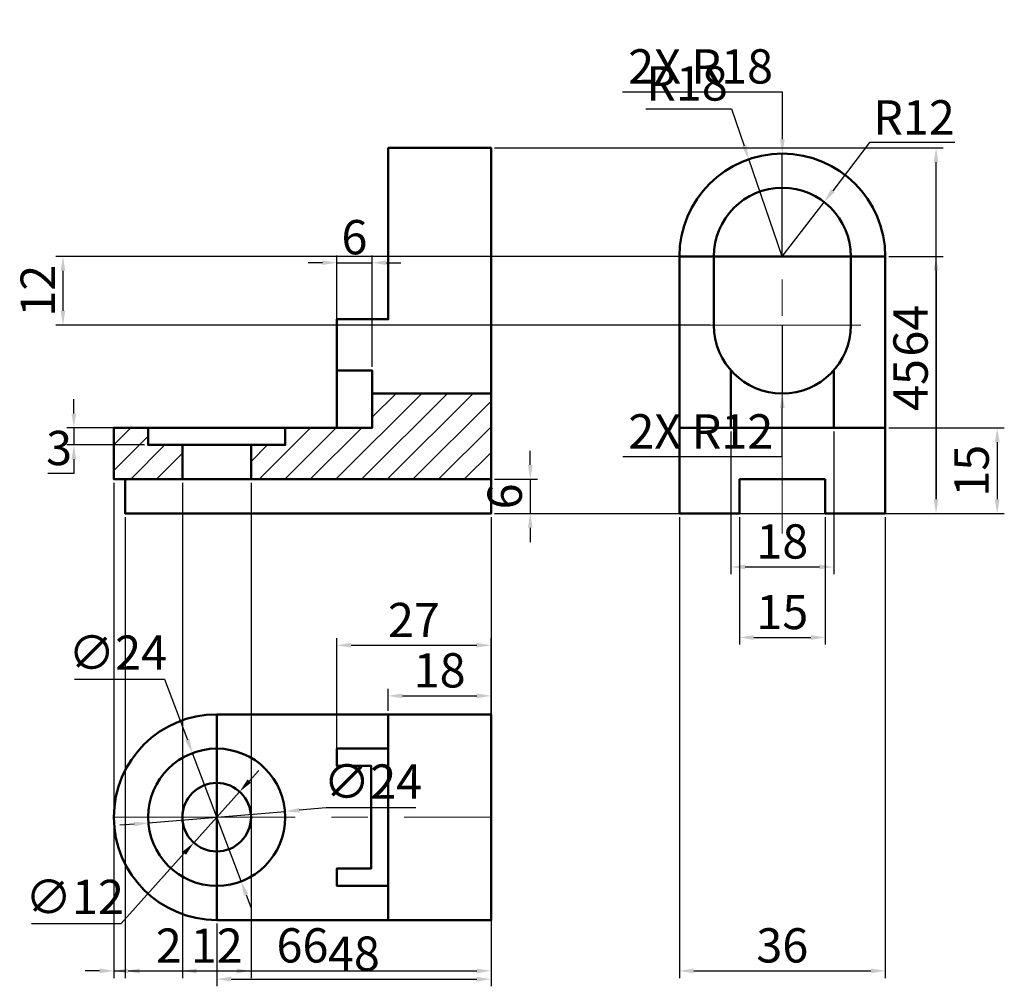
# Model space of a CAD drawing. Units: millimetres. Extents: x 1 to 173, y 26 to 195.
import ezdxf

# ---------------------------------------------------------------- set-up
doc = ezdxf.new("R2010")
doc.units = ezdxf.units.MM
doc.linetypes.add('CENTER', pattern=[50.8, 31.75, -6.35, 6.35, -6.35])
for name, color, linetype, lineweight in [('M-CNTR', 4, 'CENTER', 18), ('M-DIMS', 2, 'Continuous', 25), ('M-HATC', 8, 'Continuous', 18), ('M-OUTL', 7, 'Continuous', 50)]:
    doc.layers.add(name, color=color, linetype=linetype, lineweight=lineweight)
doc.styles.get("Standard").update_dxf_attribs({"font": 'arial.ttf'})
doc.dimstyles.new('ISO-25', dxfattribs={"dimtxt": 6, "dimasz": 2.5, "dimexe": 1.25, "dimexo": 0.625, "dimtad": 1, "dimtoh": 1, "dimdec": 0, "dimtxsty": 'Standard', "dimcen": 2.5, "dimadec": 0, "dimazin": 0, "dimtfac": 1, "dimtdec": 0, "dimtmove": 0, "dimatfit": 3, "dimfxl": 1, "dimarcsym": 0})

# ---------------------------------------------------------------- blocks, each defined once
blk = doc.blocks.new('*D1')
at = {"layer": 'Defpoints', "color": 0, "transparency": 16777216}
for p in [(62.71, 152.66), (56.52, 133.82), (62.71, 133.82)]:
    blk.add_point(p, dxfattribs=at)
at = {"layer": 'M-DIMS', "color": 0, "lineweight": -2, "transparency": 16777216}
for p, q in [((56.52, 134.44), (56.52, 153.91)), ((62.71, 134.44), (62.71, 153.91)), ((54.02, 152.66), (51.52, 152.66)), ((56.52, 152.66), (62.71, 152.66)), ((65.21, 152.66), (67.71, 152.66))]:
    blk.add_line(p, q, dxfattribs=at)
at = {"layer": 'M-DIMS', "color": 0, "transparency": 16777216}
for points in [[(54.02, 153.08), (54.02, 152.25), (56.52, 152.66)], [(65.21, 153.08), (65.21, 152.25), (62.71, 152.66)]]:
    blk.add_solid(points, dxfattribs=at)
at = {"layer": 'M-DIMS', "color": 0, "transparency": 16777216, "insert": (59.61, 156.35), "char_height": 6, "attachment_point": 5}
blk.add_mtext('6', dxfattribs=at)
blk = doc.blocks.new('*D2')
at = {"layer": 'Defpoints', "color": 0, "transparency": 16777216}
for p in [(83.52, 114.76), (83.52, 108.76), (90.38, 108.76)]:
    blk.add_point(p, dxfattribs=at)
at = {"layer": 'M-DIMS', "color": 0, "lineweight": -2, "transparency": 16777216}
for p, q in [((90.38, 117.26), (90.38, 119.76)), ((84.15, 114.76), (91.63, 114.76)), ((90.38, 114.76), (90.38, 108.76)), ((84.15, 108.76), (91.63, 108.76)), ((90.38, 106.26), (90.38, 103.76))]:
    blk.add_line(p, q, dxfattribs=at)
at = {"layer": 'M-DIMS', "color": 0, "transparency": 16777216}
for points in [[(89.96, 117.26), (90.79, 117.26), (90.38, 114.76)], [(89.96, 106.26), (90.79, 106.26), (90.38, 108.76)]]:
    blk.add_solid(points, dxfattribs=at)
at = {"layer": 'M-DIMS', "color": 0, "transparency": 16777216, "insert": (86.69, 111.76), "char_height": 6, "attachment_point": 5, "rotation": 90}
blk.add_mtext('6', dxfattribs=at)
blk = doc.blocks.new('*D3')
at = {"layer": 'Defpoints', "color": 0, "transparency": 16777216}
for p in [(23.52, 123.76), (10.53, 120.76), (23.52, 120.76)]:
    blk.add_point(p, dxfattribs=at)
at = {"layer": 'M-DIMS', "color": 0, "lineweight": -2, "transparency": 16777216}
for p, q in [((10.53, 126.26), (10.53, 128.76)), ((22.9, 123.76), (9.28, 123.76)), ((10.53, 123.76), (10.53, 120.76)), ((22.9, 120.76), (9.28, 120.76)), ((10.53, 118.26), (10.53, 115.76)), ((10.53, 115.76), (5.97, 115.76))]:
    blk.add_line(p, q, dxfattribs=at)
at = {"layer": 'M-DIMS', "color": 0, "transparency": 16777216}
for points in [[(10.11, 126.26), (10.94, 126.26), (10.53, 123.76)], [(10.11, 118.26), (10.94, 118.26), (10.53, 120.76)]]:
    blk.add_solid(points, dxfattribs=at)
at = {"layer": 'M-DIMS', "color": 0, "transparency": 16777216, "insert": (7.94, 119.45), "char_height": 6, "attachment_point": 5}
blk.add_mtext('3', dxfattribs=at)
blk = doc.blocks.new('*D4')
at = {"layer": 'Defpoints', "color": 0, "transparency": 16777216}
for p in [(128.62, 170.77), (134.48, 153.75)]:
    blk.add_point(p, dxfattribs=at)
at = {"layer": 'M-DIMS', "color": 0, "lineweight": -2, "transparency": 16777216}
for p, q in [((110.62, 179.56), (125.6, 179.56)), ((125.6, 179.56), (127.81, 173.14)), ((134.48, 153.75), (128.62, 170.77))]:
    blk.add_line(p, q, dxfattribs=at)
at = {"layer": 'M-DIMS', "color": 0, "transparency": 16777216}
blk.add_solid([(128.2, 173.27), (127.42, 173), (128.62, 170.77)], dxfattribs=at)
at = {"layer": 'M-DIMS', "color": 0, "transparency": 16777216, "insert": (117.8, 183.25), "char_height": 6, "attachment_point": 5}
blk.add_mtext('R18', dxfattribs=at)
blk = doc.blocks.new('*D5')
at = {"layer": 'Defpoints', "color": 0, "transparency": 16777216}
for p in [(141.79, 163.27), (134.48, 153.75)]:
    blk.add_point(p, dxfattribs=at)
at = {"layer": 'M-DIMS', "color": 0, "lineweight": -2, "transparency": 16777216}
for p, q in [((149.76, 173.67), (143.31, 165.26)), ((164.66, 173.67), (149.76, 173.67)), ((134.48, 153.75), (141.79, 163.27))]:
    blk.add_line(p, q, dxfattribs=at)
at = {"layer": 'M-DIMS', "color": 0, "transparency": 16777216}
blk.add_solid([(142.98, 165.51), (143.64, 165), (141.79, 163.27)], dxfattribs=at)
at = {"layer": 'M-DIMS', "color": 0, "transparency": 16777216, "insert": (157.52, 177.31), "char_height": 6, "attachment_point": 5}
blk.add_mtext('R12', dxfattribs=at)
blk = doc.blocks.new('*D6')
at = {"layer": 'Defpoints', "color": 0, "transparency": 16777216}
for p in [(152.48, 153.75), (152.48, 108.75), (161.37, 108.75)]:
    blk.add_point(p, dxfattribs=at)
at = {"layer": 'M-DIMS', "color": 0, "lineweight": -2, "transparency": 16777216}
for p, q in [((153.11, 153.75), (162.62, 153.75)), ((161.37, 151.25), (161.37, 111.25)), ((153.11, 108.75), (162.62, 108.75))]:
    blk.add_line(p, q, dxfattribs=at)
at = {"layer": 'M-DIMS', "color": 0, "transparency": 16777216}
for points in [[(160.96, 151.25), (161.79, 151.25), (161.37, 153.75)], [(160.96, 111.25), (161.79, 111.25), (161.37, 108.75)]]:
    blk.add_solid(points, dxfattribs=at)
at = {"layer": 'M-DIMS', "color": 0, "transparency": 16777216, "insert": (157.7, 131.25), "char_height": 6, "attachment_point": 5, "rotation": 90}
blk.add_mtext('45', dxfattribs=at)
blk = doc.blocks.new('*D7')
at = {"layer": 'Defpoints', "color": 0, "transparency": 16777216}
for p in [(152.48, 123.75), (152.48, 108.75), (172.07, 108.75)]:
    blk.add_point(p, dxfattribs=at)
at = {"layer": 'M-DIMS', "color": 0, "lineweight": -2, "transparency": 16777216}
for p, q in [((153.11, 123.75), (173.32, 123.75)), ((172.07, 121.25), (172.07, 111.25)), ((153.11, 108.75), (173.32, 108.75))]:
    blk.add_line(p, q, dxfattribs=at)
at = {"layer": 'M-DIMS', "color": 0, "transparency": 16777216}
for points in [[(171.65, 121.25), (172.49, 121.25), (172.07, 123.75)], [(171.65, 111.25), (172.49, 111.25), (172.07, 108.75)]]:
    blk.add_solid(points, dxfattribs=at)
at = {"layer": 'M-DIMS', "color": 0, "transparency": 16777216, "insert": (168.38, 116.25), "char_height": 6, "attachment_point": 5, "rotation": 90}
blk.add_mtext('15', dxfattribs=at)
blk = doc.blocks.new('*D8')
at = {"layer": 'Defpoints', "color": 0, "transparency": 16777216}
for p in [(126.98, 108.75), (141.98, 108.75), (141.98, 87.07)]:
    blk.add_point(p, dxfattribs=at)
at = {"layer": 'M-DIMS', "color": 0, "lineweight": -2, "transparency": 16777216}
for p, q in [((126.98, 108.13), (126.98, 85.82)), ((141.98, 108.13), (141.98, 85.82)), ((129.48, 87.07), (139.48, 87.07))]:
    blk.add_line(p, q, dxfattribs=at)
at = {"layer": 'M-DIMS', "color": 0, "transparency": 16777216}
for points in [[(129.48, 87.48), (129.48, 86.65), (126.98, 87.07)], [(139.48, 87.48), (139.48, 86.65), (141.98, 87.07)]]:
    blk.add_solid(points, dxfattribs=at)
at = {"layer": 'M-DIMS', "color": 0, "transparency": 16777216, "insert": (134.48, 90.75), "char_height": 6, "attachment_point": 5}
blk.add_mtext('15', dxfattribs=at)
blk = doc.blocks.new('*D9')
at = {"layer": 'Defpoints', "color": 0, "transparency": 16777216}
for p in [(125.48, 123.75), (143.48, 123.75), (143.48, 99.41)]:
    blk.add_point(p, dxfattribs=at)
at = {"layer": 'M-DIMS', "color": 0, "lineweight": -2, "transparency": 16777216}
for p, q in [((125.48, 123.13), (125.48, 98.16)), ((143.48, 123.13), (143.48, 98.16)), ((127.98, 99.41), (140.98, 99.41))]:
    blk.add_line(p, q, dxfattribs=at)
at = {"layer": 'M-DIMS', "color": 0, "transparency": 16777216}
for points in [[(127.98, 99.83), (127.98, 99), (125.48, 99.41)], [(140.98, 99.83), (140.98, 99), (143.48, 99.41)]]:
    blk.add_solid(points, dxfattribs=at)
at = {"layer": 'M-DIMS', "color": 0, "transparency": 16777216, "insert": (134.48, 103.1), "char_height": 6, "attachment_point": 5}
blk.add_mtext('18', dxfattribs=at)
blk = doc.blocks.new('*D10')
at = {"layer": 'Defpoints', "color": 0, "transparency": 16777216}
for p in [(83.52, 85.71), (56.52, 66.12), (83.52, 66.12)]:
    blk.add_point(p, dxfattribs=at)
at = {"layer": 'M-DIMS', "color": 0, "lineweight": -2, "transparency": 16777216}
for p, q in [((56.52, 66.74), (56.52, 86.96)), ((83.52, 66.74), (83.52, 86.96)), ((59.02, 85.71), (81.02, 85.71))]:
    blk.add_line(p, q, dxfattribs=at)
at = {"layer": 'M-DIMS', "color": 0, "transparency": 16777216}
for points in [[(59.02, 86.13), (59.02, 85.3), (56.52, 85.71)], [(81.02, 86.13), (81.02, 85.3), (83.52, 85.71)]]:
    blk.add_solid(points, dxfattribs=at)
at = {"layer": 'M-DIMS', "color": 0, "transparency": 16777216, "insert": (70.02, 89.35), "char_height": 6, "attachment_point": 5}
blk.add_mtext('27', dxfattribs=at)
blk = doc.blocks.new('*D11')
at = {"layer": 'Defpoints', "color": 0, "transparency": 16777216}
for p in [(83.52, 76.85), (65.52, 73.62), (83.52, 73.62)]:
    blk.add_point(p, dxfattribs=at)
at = {"layer": 'M-DIMS', "color": 0, "lineweight": -2, "transparency": 16777216}
for p, q in [((65.52, 74.24), (65.52, 78.1)), ((83.52, 74.24), (83.52, 78.1)), ((68.02, 76.85), (81.02, 76.85))]:
    blk.add_line(p, q, dxfattribs=at)
at = {"layer": 'M-DIMS', "color": 0, "transparency": 16777216}
for points in [[(68.02, 77.27), (68.02, 76.44), (65.52, 76.85)], [(81.02, 77.27), (81.02, 76.44), (83.52, 76.85)]]:
    blk.add_solid(points, dxfattribs=at)
at = {"layer": 'M-DIMS', "color": 0, "transparency": 16777216, "insert": (74.52, 80.54), "char_height": 6, "attachment_point": 5}
blk.add_mtext('18', dxfattribs=at)
blk = doc.blocks.new('*D12')
at = {"layer": 'Defpoints', "color": 0, "transparency": 16777216}
for p in [(35.52, 37.62), (83.52, 37.62), (83.52, 27.27)]:
    blk.add_point(p, dxfattribs=at)
at = {"layer": 'M-DIMS', "color": 0, "lineweight": -2, "transparency": 16777216}
for p, q in [((35.52, 36.99), (35.52, 26.02)), ((83.52, 36.99), (83.52, 26.02)), ((38.02, 27.27), (81.02, 27.27))]:
    blk.add_line(p, q, dxfattribs=at)
at = {"layer": 'M-DIMS', "color": 0, "transparency": 16777216}
for points in [[(38.02, 27.69), (38.02, 26.86), (35.52, 27.27)], [(81.02, 27.69), (81.02, 26.86), (83.52, 27.27)]]:
    blk.add_solid(points, dxfattribs=at)
at = {"layer": 'M-DIMS', "color": 0, "transparency": 16777216, "insert": (59.52, 30.96), "char_height": 6, "attachment_point": 5}
blk.add_mtext('48', dxfattribs=at)
blk = doc.blocks.new('*D13')
at = {"layer": 'Defpoints', "color": 0, "transparency": 16777216}
for p in [(31.27, 66.84), (39.77, 44.4)]:
    blk.add_point(p, dxfattribs=at)
at = {"layer": 'M-DIMS', "color": 0, "lineweight": -2, "transparency": 16777216}
for p, q in [((10.65, 79.79), (26.37, 79.79)), ((26.37, 79.79), (30.39, 69.18)), ((39.77, 44.4), (31.27, 66.84)), ((40.66, 42.06), (41.54, 39.72))]:
    blk.add_line(p, q, dxfattribs=at)
at = {"layer": 'M-DIMS', "color": 0, "transparency": 16777216}
for points in [[(30.78, 69.33), (30, 69.03), (31.27, 66.84)], [(41.05, 42.21), (40.27, 41.91), (39.77, 44.4)]]:
    blk.add_solid(points, dxfattribs=at)
at = {"layer": 'M-DIMS', "color": 0, "transparency": 16777216, "insert": (18.2, 83.64), "char_height": 6, "attachment_point": 5}
blk.add_mtext('∅24', dxfattribs=at)
blk = doc.blocks.new('*D14')
at = {"layer": 'Defpoints', "color": 0, "transparency": 16777216}
for p in [(39.53, 60.08), (31.51, 51.16)]:
    blk.add_point(p, dxfattribs=at)
at = {"layer": 'M-DIMS', "color": 0, "lineweight": -2, "transparency": 16777216}
for p, q in [((41.21, 61.94), (42.88, 63.8)), ((39.53, 60.08), (31.51, 51.16)), ((18.81, 37.04), (29.84, 49.3)), ((3.12, 37.04), (18.81, 37.04))]:
    blk.add_line(p, q, dxfattribs=at)
at = {"layer": 'M-DIMS', "color": 0, "transparency": 16777216}
for points in [[(40.9, 62.22), (41.51, 61.66), (39.53, 60.08)], [(29.53, 49.58), (30.15, 49.02), (31.51, 51.16)]]:
    blk.add_solid(points, dxfattribs=at)
at = {"layer": 'M-DIMS', "color": 0, "transparency": 16777216, "insert": (10.65, 40.89), "char_height": 6, "attachment_point": 5}
blk.add_mtext('∅12', dxfattribs=at)
blk = doc.blocks.new('*D15')
at = {"layer": 'Defpoints', "color": 0, "transparency": 16777216}
for p in [(17.52, 114.76), (83.52, 108.76), (83.52, 28.72)]:
    blk.add_point(p, dxfattribs=at)
at = {"layer": 'M-DIMS', "color": 0, "lineweight": -2, "transparency": 16777216}
for p, q in [((17.52, 114.13), (17.52, 27.47)), ((83.52, 108.13), (83.52, 27.47)), ((20.02, 28.72), (81.02, 28.72))]:
    blk.add_line(p, q, dxfattribs=at)
at = {"layer": 'M-DIMS', "color": 0, "transparency": 16777216}
for points in [[(20.02, 29.14), (20.02, 28.3), (17.52, 28.72)], [(81.02, 29.14), (81.02, 28.3), (83.52, 28.72)]]:
    blk.add_solid(points, dxfattribs=at)
at = {"layer": 'M-DIMS', "color": 0, "transparency": 16777216, "insert": (50.52, 32.41), "char_height": 6, "attachment_point": 5}
blk.add_mtext('66', dxfattribs=at)
blk = doc.blocks.new('*D16')
at = {"layer": 'Defpoints', "color": 0, "transparency": 16777216}
for p in [(116.48, 108.75), (152.48, 108.75), (152.48, 28.72)]:
    blk.add_point(p, dxfattribs=at)
at = {"layer": 'M-DIMS', "color": 0, "lineweight": -2, "transparency": 16777216}
for p, q in [((116.48, 108.13), (116.48, 27.47)), ((152.48, 108.13), (152.48, 27.47)), ((118.98, 28.72), (149.98, 28.72))]:
    blk.add_line(p, q, dxfattribs=at)
at = {"layer": 'M-DIMS', "color": 0, "transparency": 16777216}
for points in [[(118.98, 29.14), (118.98, 28.3), (116.48, 28.72)], [(149.98, 29.14), (149.98, 28.3), (152.48, 28.72)]]:
    blk.add_solid(points, dxfattribs=at)
at = {"layer": 'M-DIMS', "color": 0, "transparency": 16777216, "insert": (134.48, 32.41), "char_height": 6, "attachment_point": 5}
blk.add_mtext('36', dxfattribs=at)
blk = doc.blocks.new('*D17')
at = {"layer": 'Defpoints', "color": 0, "transparency": 16777216}
for p in [(83.52, 172.75), (161.38, 172.75), (83.52, 108.76)]:
    blk.add_point(p, dxfattribs=at)
at = {"layer": 'M-DIMS', "color": 0, "lineweight": -2, "transparency": 16777216}
for p, q in [((84.15, 172.75), (162.63, 172.75)), ((161.38, 111.26), (161.38, 170.25)), ((84.15, 108.76), (162.63, 108.76))]:
    blk.add_line(p, q, dxfattribs=at)
at = {"layer": 'M-DIMS', "color": 0, "transparency": 16777216}
for points in [[(160.97, 170.25), (161.8, 170.25), (161.38, 172.75)], [(160.97, 111.26), (161.8, 111.26), (161.38, 108.76)]]:
    blk.add_solid(points, dxfattribs=at)
at = {"layer": 'M-DIMS', "color": 0, "transparency": 16777216, "insert": (157.69, 140.76), "char_height": 6, "attachment_point": 5, "rotation": 90}
blk.add_mtext('64', dxfattribs=at)
blk = doc.blocks.new('*D18')
at = {"layer": 'Defpoints', "color": 0, "transparency": 16777216}
for p in [(122.48, 153.75), (8.62, 141.75), (122.48, 141.75)]:
    blk.add_point(p, dxfattribs=at)
at = {"layer": 'M-DIMS', "color": 0, "lineweight": -2, "transparency": 16777216}
for p, q in [((121.86, 153.75), (7.37, 153.75)), ((8.62, 151.25), (8.62, 144.25)), ((121.86, 141.75), (7.37, 141.75))]:
    blk.add_line(p, q, dxfattribs=at)
at = {"layer": 'M-DIMS', "color": 0, "transparency": 16777216}
for points in [[(8.2, 151.25), (9.04, 151.25), (8.62, 153.75)], [(8.2, 144.25), (9.04, 144.25), (8.62, 141.75)]]:
    blk.add_solid(points, dxfattribs=at)
at = {"layer": 'M-DIMS', "color": 0, "transparency": 16777216, "insert": (4.98, 147.75), "char_height": 6, "attachment_point": 5, "rotation": 90}
blk.add_mtext('12', dxfattribs=at)
blk = doc.blocks.new('*D19')
at = {"layer": 'Defpoints', "color": 0, "transparency": 16777216}
for p in [(17.52, 114.76), (19.52, 108.76), (19.52, 28.72)]:
    blk.add_point(p, dxfattribs=at)
at = {"layer": 'M-DIMS', "color": 0, "lineweight": -2, "transparency": 16777216}
for p, q in [((17.52, 114.13), (17.52, 27.47)), ((19.52, 108.13), (19.52, 27.47)), ((15.02, 28.72), (12.52, 28.72)), ((17.52, 28.72), (19.52, 28.72)), ((22.02, 28.72), (29.74, 28.72))]:
    blk.add_line(p, q, dxfattribs=at)
at = {"layer": 'M-DIMS', "color": 0, "transparency": 16777216}
for points in [[(15.02, 29.14), (15.02, 28.3), (17.52, 28.72)], [(22.02, 29.14), (22.02, 28.3), (19.52, 28.72)]]:
    blk.add_solid(points, dxfattribs=at)
at = {"layer": 'M-DIMS', "color": 0, "transparency": 16777216, "insert": (27.13, 32.36), "char_height": 6, "attachment_point": 5}
blk.add_mtext('2', dxfattribs=at)
blk = doc.blocks.new('*D20')
at = {"layer": 'Defpoints', "color": 0, "transparency": 16777216}
for p in [(29.52, 114.76), (41.52, 114.76), (41.52, 28.72)]:
    blk.add_point(p, dxfattribs=at)
at = {"layer": 'M-DIMS', "color": 0, "lineweight": -2, "transparency": 16777216}
for p, q in [((29.52, 114.13), (29.52, 27.47)), ((41.52, 114.13), (41.52, 27.47)), ((32.02, 28.72), (39.02, 28.72))]:
    blk.add_line(p, q, dxfattribs=at)
at = {"layer": 'M-DIMS', "color": 0, "transparency": 16777216}
for points in [[(32.02, 29.14), (32.02, 28.3), (29.52, 28.72)], [(39.02, 29.14), (39.02, 28.3), (41.52, 28.72)]]:
    blk.add_solid(points, dxfattribs=at)
at = {"layer": 'M-DIMS', "color": 0, "transparency": 16777216, "insert": (35.52, 32.36), "char_height": 6, "attachment_point": 5}
blk.add_mtext('12', dxfattribs=at)
blk = doc.blocks.new('*D21')
at = {"layer": 'Defpoints', "color": 0, "transparency": 16777216}
for p in [(134.48, 171.75), (134.48, 153.75)]:
    blk.add_point(p, dxfattribs=at)
at = {"layer": 'M-DIMS', "color": 0, "lineweight": -2, "transparency": 16777216}
for p, q in [((106.51, 182.55), (134.48, 182.55)), ((134.48, 182.55), (134.48, 174.25)), ((134.48, 153.75), (134.48, 171.75))]:
    blk.add_line(p, q, dxfattribs=at)
at = {"layer": 'M-DIMS', "color": 0, "transparency": 16777216}
blk.add_solid([(134.9, 174.25), (134.07, 174.25), (134.48, 171.75)], dxfattribs=at)
at = {"layer": 'M-DIMS', "color": 0, "transparency": 16777216, "insert": (120.18, 186.24), "char_height": 6, "attachment_point": 5}
blk.add_mtext('2X R18', dxfattribs=at)
blk = doc.blocks.new('*D22')
at = {"layer": 'Defpoints', "color": 0, "transparency": 16777216}
for p in [(134.48, 141.75), (134.48, 129.75)]:
    blk.add_point(p, dxfattribs=at)
at = {"layer": 'M-DIMS', "color": 0, "lineweight": -2, "transparency": 16777216}
for p, q in [((134.48, 141.75), (134.48, 129.75)), ((134.48, 118.72), (134.48, 127.25)), ((106.59, 118.72), (134.48, 118.72))]:
    blk.add_line(p, q, dxfattribs=at)
at = {"layer": 'M-DIMS', "color": 0, "transparency": 16777216}
blk.add_solid([(134.07, 127.25), (134.9, 127.25), (134.48, 129.75)], dxfattribs=at)
at = {"layer": 'M-DIMS', "color": 0, "transparency": 16777216, "insert": (120.22, 122.36), "char_height": 6, "attachment_point": 5}
blk.add_mtext('2X R12', dxfattribs=at)
blk = doc.blocks.new('*D23')
at = {"layer": 'Defpoints', "color": 0, "transparency": 16777216}
for p in [(47.48, 56.62), (23.56, 54.61)]:
    blk.add_point(p, dxfattribs=at)
at = {"layer": 'M-DIMS', "color": 0, "lineweight": -2, "transparency": 16777216}
for p, q in [((54.65, 57.23), (49.97, 56.83)), ((70.38, 57.23), (54.65, 57.23)), ((23.56, 54.61), (47.48, 56.62)), ((21.07, 54.4), (18.58, 54.2))]:
    blk.add_line(p, q, dxfattribs=at)
at = {"layer": 'M-DIMS', "color": 0, "transparency": 16777216}
for points in [[(49.94, 57.25), (50, 56.42), (47.48, 56.62)], [(21.04, 54.82), (21.11, 53.99), (23.56, 54.61)]]:
    blk.add_solid(points, dxfattribs=at)
at = {"layer": 'M-DIMS', "color": 0, "transparency": 16777216, "insert": (62.83, 61.08), "char_height": 6, "attachment_point": 5}
blk.add_mtext('∅24', dxfattribs=at)

msp = doc.modelspace()

# ---------------------------------------------------------------- hatches: boundary and pattern name
at = {"layer": 'M-HATC'}
h = msp.add_hatch(dxfattribs=at)
h.set_pattern_fill('ANSI31', color=256)
h.paths.add_polyline_path([(83.52, 129.76), (62.74, 129.76), (62.74, 123.76), (47.52, 123.76), (47.52, 120.76), (41.52, 120.76), (41.52, 114.76), (83.52, 114.76)])
h.paths.add_polyline_path([(29.52, 120.76), (23.52, 120.76), (23.52, 123.76), (17.52, 123.76), (17.52, 114.76), (19.52, 114.76), (29.52, 114.76)])

# ---------------------------------------------------------------- linework, layer by layer
at = {"layer": 'M-CNTR'}
for p, q in [((134.48, 105.25), (134.48, 157.25)), ((116.48, 141.75), (152.48, 141.75)), ((17.52, 55.62), (83.52, 55.62))]:
    msp.add_line(p, q, dxfattribs=at)
at = {"layer": 'M-OUTL'}
for p, q in [((116.48, 108.75), (116.48, 153.75)), ((152.48, 108.75), (152.48, 153.75)), ((125.48, 123.75), (125.48, 133.82)), ((143.48, 123.75), (143.48, 133.82)), ((134.48, 129.75), (134.48, 129.75)), ((116.48, 123.75), (152.48, 123.75)), ((29.52, 114.76), (29.52, 120.76)), ((41.52, 114.76), (41.52, 120.76)), ((126.98, 108.75), (126.98, 114.75)), ((126.98, 114.75), (141.98, 114.75)), ((141.98, 114.75), (141.98, 108.75)), ((116.48, 108.75), (126.98, 108.75)), ((141.98, 108.75), (152.48, 108.75)), ((83.52, 73.62), (35.52, 73.62)), ((65.52, 37.62), (65.52, 73.62)), ((83.52, 37.62), (83.52, 73.62)), ((35.52, 37.62), (83.52, 37.62))]:
    msp.add_line(p, q, dxfattribs=at)
for points in [[(83.52, 129.76), (83.52, 172.75), (65.52, 172.75), (65.52, 142.75), (56.52, 142.75), (56.52, 123.76)], [(56.52, 133.82), (62.71, 133.82), (62.71, 129.76), (83.52, 129.76), (83.52, 108.76), (19.52, 108.76), (19.52, 114.76)], [(62.74, 129.76), (62.74, 123.76), (17.52, 123.76), (17.52, 114.76), (19.52, 114.76), (83.52, 114.76)], [(23.52, 123.76), (23.52, 120.76), (47.52, 120.76), (47.52, 123.76)], [(65.52, 43.62), (56.52, 43.62), (56.52, 46.62), (62.52, 46.62), (62.52, 64.62), (56.52, 64.62), (56.52, 67.62), (65.52, 67.62)]]:
    msp.add_lwpolyline(points, dxfattribs=at)
for points in [[(152.48, 153.75, 1), (116.48, 153.75)], [(146.48, 153.75), (146.48, 141.75, -1), (122.48, 141.75), (122.48, 153.75, -1)], [(35.52, 73.62, 1), (35.52, 37.62)]]:
    msp.add_lwpolyline(points, format="xyb", close=True, dxfattribs=at)
for radius in [12, 6]:
    msp.add_circle((35.52, 55.62), radius, dxfattribs=at)

# ---------------------------------------------------------------- dimensions: what is measured, and where the dimension line sits
at = {"layer": 'M-DIMS'}
dim = msp.add_radius_dim(center=(134.48, 153.75), mpoint=(134.48, 171.75), text='2X <>', dimstyle='ISO-25', override={"dimdec": 0, "dimlfac": 1, "dimrnd": 0, "dimzin": 0, "dimdsep": 46, "dimlunit": 2}, dxfattribs=at)
dim.commit()
dim.dimension.update_dxf_attribs({"geometry": '*D21', "text_midpoint": (120.18, 182.55), "dimtype": 164})
for mpoint, picture, middle in [((128.62, 170.77), '*D4', (117.8, 179.56)), ((141.79, 163.27), '*D5', (157.52, 173.67))]:
    dim = msp.add_radius_dim(center=(134.48, 153.75), mpoint=mpoint, dimstyle='ISO-25', override={"dimclrd": 0, "dimclre": 0, "dimclrt": 0}, dxfattribs=at)
    dim.commit()
    dim.dimension.update_dxf_attribs({"geometry": picture, "text_midpoint": middle, "dimtype": 164})
for base, p1, p2, override, picture, middle in [((161.38, 172.75), (83.52, 108.76), (83.52, 172.75), {"dimdec": 0, "dimlfac": 1, "dimrnd": 0, "dimzin": 0, "dimdsep": 46, "dimlunit": 2}, '*D17', (157.69, 140.76)), ((8.62, 141.75), (122.48, 153.75), (122.48, 141.75), {"dimdec": 0, "dimlfac": 1, "dimrnd": 0, "dimzin": 0, "dimdsep": 46, "dimlunit": 2}, '*D18', (4.98, 147.75)), ((161.37, 108.75), (152.48, 153.75), (152.48, 108.75), {"dimclrd": 0, "dimclre": 0, "dimclrt": 0}, '*D6', (157.7, 131.25)), ((10.53, 120.76), (23.52, 123.76), (23.52, 120.76), {"dimclrd": 0, "dimclre": 0, "dimclrt": 0}, '*D3', (7.94, 119.45)), ((172.07, 108.75), (152.48, 123.75), (152.48, 108.75), {"dimclrd": 0, "dimclre": 0, "dimclrt": 0}, '*D7', (168.38, 116.25)), ((90.38, 108.76), (83.52, 114.76), (83.52, 108.76), {"dimclrd": 0, "dimclre": 0, "dimclrt": 0}, '*D2', (86.69, 111.76))]:
    dim = msp.add_linear_dim(base=base, p1=p1, p2=p2, angle=90, dimstyle='ISO-25', override=override, dxfattribs=at)
    dim.commit()
    dim.dimension.update_dxf_attribs({"geometry": picture, "text_midpoint": middle})
for base, p1, p2, override, picture, middle in [((62.71, 152.66), (56.52, 133.82), (62.71, 133.82), {"dimclrd": 0, "dimclre": 0, "dimclrt": 0}, '*D1', (59.61, 156.35)), ((143.48, 99.41), (125.48, 123.75), (143.48, 123.75), {"dimclrd": 0, "dimclre": 0, "dimclrt": 0}, '*D9', (134.48, 103.1)), ((19.52, 28.72), (17.52, 114.76), (19.52, 108.76), {"dimdec": 0, "dimlfac": 1, "dimrnd": 0, "dimzin": 0, "dimdsep": 46, "dimlunit": 2}, '*D19', (27.13, 32.36)), ((83.52, 28.72), (17.52, 114.76), (83.52, 108.76), {"dimdec": 0, "dimlfac": 1, "dimrnd": 0, "dimzin": 0, "dimdsep": 46, "dimlunit": 2}, '*D15', (50.52, 32.41)), ((41.52, 28.72), (29.52, 114.76), (41.52, 114.76), {"dimdec": 0, "dimlfac": 1, "dimrnd": 0, "dimzin": 0, "dimdsep": 46, "dimlunit": 2}, '*D20', (35.52, 32.36)), ((152.48, 28.72), (116.48, 108.75), (152.48, 108.75), {"dimdec": 0, "dimlfac": 1, "dimrnd": 0, "dimzin": 0, "dimdsep": 46, "dimlunit": 2}, '*D16', (134.48, 32.41)), ((141.98, 87.07), (126.98, 108.75), (141.98, 108.75), {"dimclrd": 0, "dimclre": 0, "dimclrt": 0}, '*D8', (134.48, 90.75)), ((83.52, 85.71), (56.52, 66.12), (83.52, 66.12), {"dimclrd": 0, "dimclre": 0, "dimclrt": 0}, '*D10', (70.02, 89.35)), ((83.52, 76.85), (65.52, 73.62), (83.52, 73.62), {"dimclrd": 0, "dimclre": 0, "dimclrt": 0}, '*D11', (74.52, 80.54)), ((83.52, 27.27), (35.52, 37.62), (83.52, 37.62), {"dimclrd": 0, "dimclre": 0, "dimclrt": 0}, '*D12', (59.52, 30.96))]:
    dim = msp.add_linear_dim(base=base, p1=p1, p2=p2, dimstyle='ISO-25', override=override, dxfattribs=at)
    dim.commit()
    dim.dimension.update_dxf_attribs({"geometry": picture, "text_midpoint": middle})
dim = msp.add_radius_dim(center=(134.48, 141.75), mpoint=(134.48, 129.75), text='2X <>', dimstyle='ISO-25', override={"dimdec": 0, "dimlfac": 1, "dimrnd": 0, "dimzin": 0, "dimdsep": 46, "dimlunit": 2}, dxfattribs=at)
dim.commit()
dim.dimension.update_dxf_attribs({"geometry": '*D22', "text_midpoint": (120.22, 122.36)})
for p1, p2, override, picture, middle in [((39.77, 44.4), (31.27, 66.84), {"dimclrd": 0, "dimclre": 0, "dimclrt": 0}, '*D13', (18.2, 79.79)), ((39.53, 60.08), (31.51, 51.16), {"dimclrd": 0, "dimclre": 0, "dimclrt": 0}, '*D14', (10.65, 37.04)), ((23.56, 54.61), (47.48, 56.62), {"dimdec": 0, "dimlfac": 1, "dimrnd": 0, "dimzin": 0, "dimdsep": 46, "dimlunit": 2}, '*D23', (54.65, 57.23))]:
    dim = msp.add_diameter_dim_2p(p1=p1, p2=p2, dimstyle='ISO-25', override=override, dxfattribs=at)
    dim.commit()
    dim.dimension.update_dxf_attribs({"geometry": picture, "text_midpoint": middle, "dimtype": 163})

doc.saveas('drawing.dxf')
